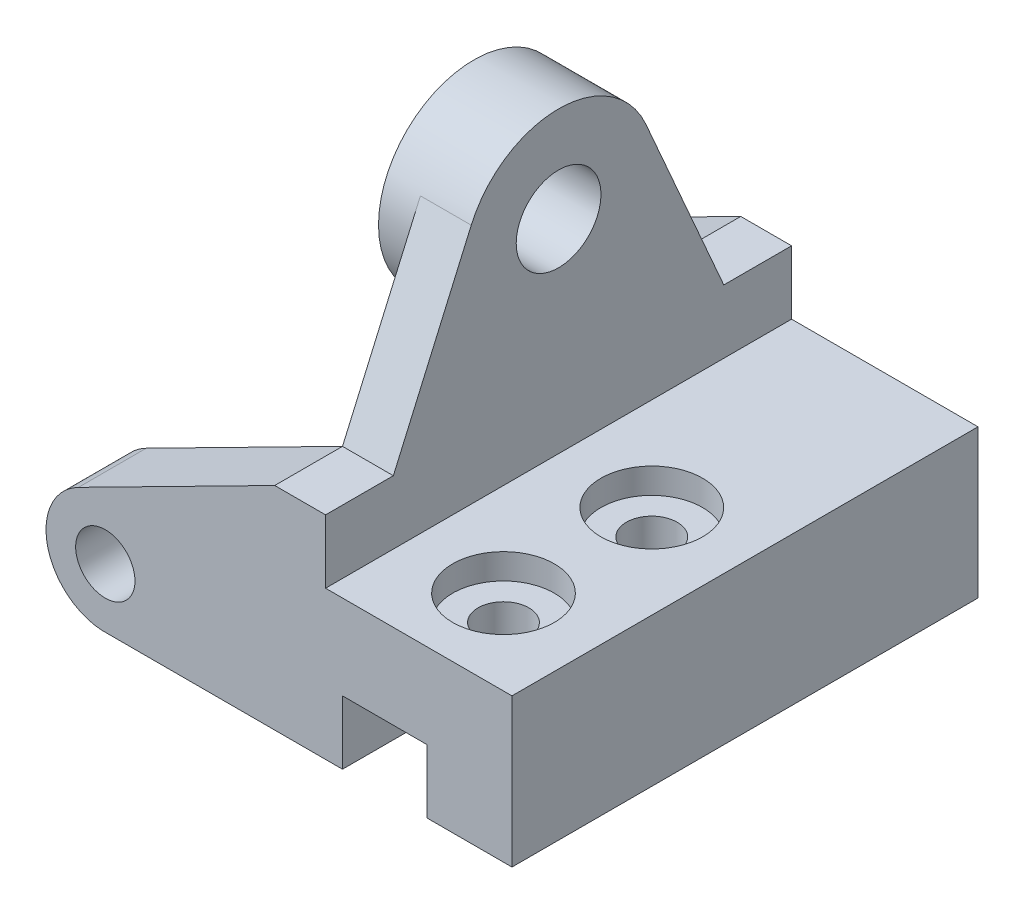
ISO-10303-21;
HEADER;
FILE_DESCRIPTION(('STEP AP214'),'2;1');
FILE_NAME('part.step','',(''),(''),'','','');
FILE_SCHEMA(('AUTOMOTIVE_DESIGN { 1 0 10303 214 1 1 1 1 }'));
ENDSEC;
DATA;
#1=APPLICATION_CONTEXT('core data for automotive mechanical design processes');
#2=APPLICATION_PROTOCOL_DEFINITION('international standard','automotive_design',2000,#1);
#3=PRODUCT_CONTEXT('',#1,'mechanical');
#4=PRODUCT('Part','Part','',(#3));
#5=PRODUCT_RELATED_PRODUCT_CATEGORY('part','',(#4));
#6=PRODUCT_DEFINITION_FORMATION('','',#4);
#7=PRODUCT_DEFINITION_CONTEXT('part definition',#1,'design');
#8=PRODUCT_DEFINITION('design','',#6,#7);
#9=PRODUCT_DEFINITION_SHAPE('','',#8);
#10=(LENGTH_UNIT() NAMED_UNIT(*) SI_UNIT(.MILLI.,.METRE.));
#11=(NAMED_UNIT(*) PLANE_ANGLE_UNIT() SI_UNIT($,.RADIAN.));
#12=(NAMED_UNIT(*) SI_UNIT($,.STERADIAN.) SOLID_ANGLE_UNIT());
#13=UNCERTAINTY_MEASURE_WITH_UNIT(LENGTH_MEASURE(1.E-05),#10,'distance_accuracy_value','');
#14=(GEOMETRIC_REPRESENTATION_CONTEXT(3) GLOBAL_UNCERTAINTY_ASSIGNED_CONTEXT((#13)) GLOBAL_UNIT_ASSIGNED_CONTEXT((#10,
#11,#12)) REPRESENTATION_CONTEXT('',''));
#15=CARTESIAN_POINT('',(0.,0.,0.));
#16=DIRECTION('',(0.,0.,1.));
#17=DIRECTION('',(1.,0.,0.));
#18=AXIS2_PLACEMENT_3D('',#15,#16,#17);
#19=CARTESIAN_POINT('',(6.,50.,0.));
#20=DIRECTION('',(0.,1.,0.));
#21=DIRECTION('',(0.,0.,1.));
#22=AXIS2_PLACEMENT_3D('',#19,#20,#21);
#23=PLANE('',#22);
#24=DIRECTION('',(0.,0.,1.));
#25=VECTOR('',#24,1.);
#26=CARTESIAN_POINT('',(6.,50.,0.));
#27=LINE('',#26,#25);
#28=CARTESIAN_POINT('',(6.,50.,94.));
#29=VERTEX_POINT('',#28);
#30=CARTESIAN_POINT('',(6.,50.,110.));
#31=VERTEX_POINT('',#30);
#32=EDGE_CURVE('E347',#29,#31,#27,.T.);
#33=ORIENTED_EDGE('',*,*,#32,.F.);
#34=DIRECTION('',(-1.,0.,0.));
#35=VECTOR('',#34,1.);
#36=CARTESIAN_POINT('',(6.,50.,94.));
#37=LINE('',#36,#35);
#38=CARTESIAN_POINT('',(-6.,50.,94.));
#39=VERTEX_POINT('',#38);
#40=EDGE_CURVE('E262',#29,#39,#37,.T.);
#41=ORIENTED_EDGE('',*,*,#40,.T.);
#42=DIRECTION('',(0.,0.,1.));
#43=VECTOR('',#42,1.);
#44=CARTESIAN_POINT('',(-6.,50.,94.));
#45=LINE('',#44,#43);
#46=CARTESIAN_POINT('',(-6.,50.,110.));
#47=VERTEX_POINT('',#46);
#48=EDGE_CURVE('E325',#39,#47,#45,.T.);
#49=ORIENTED_EDGE('',*,*,#48,.T.);
#50=DIRECTION('',(-1.,0.,0.));
#51=VECTOR('',#50,1.);
#52=CARTESIAN_POINT('',(6.,50.,110.));
#53=LINE('',#52,#51);
#54=EDGE_CURVE('E332',#31,#47,#53,.T.);
#55=ORIENTED_EDGE('',*,*,#54,.F.);
#56=EDGE_LOOP('',(#33,#41,#49,#55));
#57=FACE_BOUND('',#56,.T.);
#58=ADVANCED_FACE('F50',(#57),#23,.T.);
#59=CARTESIAN_POINT('',(-6.,35.,110.));
#60=DIRECTION('',(1.,0.,0.));
#61=DIRECTION('',(0.,0.,-1.));
#62=AXIS2_PLACEMENT_3D('',#59,#60,#61);
#63=PLANE('',#62);
#64=CARTESIAN_POINT('',(-6.,83.,55.));
#65=DIRECTION('',(-1.,0.,0.));
#66=DIRECTION('',(0.,0.,1.));
#67=AXIS2_PLACEMENT_3D('',#64,#65,#66);
#68=CIRCLE('',#67,22.5);
#69=CARTESIAN_POINT('',(-6.,92.0198235139329,34.3870724112875));
#70=VERTEX_POINT('',#69);
#71=CARTESIAN_POINT('',(-6.,92.0198235139329,75.6129275887125));
#72=VERTEX_POINT('',#71);
#73=EDGE_CURVE('E240',#70,#72,#68,.T.);
#74=ORIENTED_EDGE('',*,*,#73,.F.);
#75=DIRECTION('',(0.,-0.916130115053887,-0.400881045063684));
#76=VECTOR('',#75,1.);
#77=CARTESIAN_POINT('',(-6.,92.0198235139329,34.3870724112875));
#78=LINE('',#77,#76);
#79=CARTESIAN_POINT('',(-6.,50.,16.));
#80=VERTEX_POINT('',#79);
#81=EDGE_CURVE('E243',#70,#80,#78,.T.);
#82=ORIENTED_EDGE('',*,*,#81,.T.);
#83=DIRECTION('',(0.,-1.,0.));
#84=VECTOR('',#83,1.);
#85=CARTESIAN_POINT('',(-6.,50.,16.));
#86=LINE('',#85,#84);
#87=CARTESIAN_POINT('',(-6.,0.,16.));
#88=VERTEX_POINT('',#87);
#89=EDGE_CURVE('E278',#80,#88,#86,.T.);
#90=ORIENTED_EDGE('',*,*,#89,.T.);
#91=DIRECTION('',(0.,0.,-1.));
#92=VECTOR('',#91,1.);
#93=CARTESIAN_POINT('',(-6.,0.,110.));
#94=LINE('',#93,#92);
#95=CARTESIAN_POINT('',(-6.,0.,94.));
#96=VERTEX_POINT('',#95);
#97=EDGE_CURVE('E390',#96,#88,#94,.T.);
#98=ORIENTED_EDGE('',*,*,#97,.F.);
#99=DIRECTION('',(0.,-1.,0.));
#100=VECTOR('',#99,1.);
#101=CARTESIAN_POINT('',(-6.,0.,94.));
#102=LINE('',#101,#100);
#103=EDGE_CURVE('E313',#39,#96,#102,.T.);
#104=ORIENTED_EDGE('',*,*,#103,.F.);
#105=DIRECTION('',(0.,0.916130115053887,-0.400881045063683));
#106=VECTOR('',#105,1.);
#107=CARTESIAN_POINT('',(-6.,50.,94.));
#108=LINE('',#107,#106);
#109=EDGE_CURVE('E249',#39,#72,#108,.T.);
#110=ORIENTED_EDGE('',*,*,#109,.T.);
#111=EDGE_LOOP('',(#74,#82,#90,#98,#104,#110));
#112=FACE_BOUND('',#111,.T.);
#113=ADVANCED_FACE('F475',(#112),#63,.F.);
#114=CARTESIAN_POINT('',(-6.,0.,110.));
#115=DIRECTION('',(0.,1.,0.));
#116=DIRECTION('',(0.,0.,1.));
#117=AXIS2_PLACEMENT_3D('',#114,#115,#116);
#118=PLANE('',#117);
#119=DIRECTION('',(0.,0.,1.));
#120=VECTOR('',#119,1.);
#121=CARTESIAN_POINT('',(30.,0.,0.));
#122=LINE('',#121,#120);
#123=CARTESIAN_POINT('',(30.,0.,0.));
#124=VERTEX_POINT('',#123);
#125=CARTESIAN_POINT('',(30.,0.,110.));
#126=VERTEX_POINT('',#125);
#127=EDGE_CURVE('E366',#124,#126,#122,.T.);
#128=ORIENTED_EDGE('',*,*,#127,.F.);
#129=DIRECTION('',(1.,0.,0.));
#130=VECTOR('',#129,1.);
#131=CARTESIAN_POINT('',(-6.,0.,0.));
#132=LINE('',#131,#130);
#133=CARTESIAN_POINT('',(50.,0.,0.));
#134=VERTEX_POINT('',#133);
#135=EDGE_CURVE('E368',#124,#134,#132,.T.);
#136=ORIENTED_EDGE('',*,*,#135,.T.);
#137=DIRECTION('',(0.,0.,-1.));
#138=VECTOR('',#137,1.);
#139=CARTESIAN_POINT('',(50.,0.,110.));
#140=LINE('',#139,#138);
#141=CARTESIAN_POINT('',(50.,0.,110.));
#142=VERTEX_POINT('',#141);
#143=EDGE_CURVE('E402',#142,#134,#140,.T.);
#144=ORIENTED_EDGE('',*,*,#143,.F.);
#145=DIRECTION('',(1.,0.,0.));
#146=VECTOR('',#145,1.);
#147=CARTESIAN_POINT('',(-6.,0.,110.));
#148=LINE('',#147,#146);
#149=EDGE_CURVE('E385',#126,#142,#148,.T.);
#150=ORIENTED_EDGE('',*,*,#149,.F.);
#151=EDGE_LOOP('',(#128,#136,#144,#150));
#152=FACE_BOUND('',#151,.T.);
#153=ADVANCED_FACE('F47',(#152),#118,.F.);
#154=DIRECTION('',(0.,0.,1.));
#155=VECTOR('',#154,1.);
#156=CARTESIAN_POINT('',(10.,0.,0.));
#157=LINE('',#156,#155);
#158=CARTESIAN_POINT('',(10.,0.,0.));
#159=VERTEX_POINT('',#158);
#160=CARTESIAN_POINT('',(10.,0.,110.));
#161=VERTEX_POINT('',#160);
#162=EDGE_CURVE('E367',#159,#161,#157,.T.);
#163=ORIENTED_EDGE('',*,*,#162,.T.);
#164=CARTESIAN_POINT('',(-45.1510571856392,0.,110.));
#165=VERTEX_POINT('',#164);
#166=EDGE_CURVE('E377',#165,#161,#148,.T.);
#167=ORIENTED_EDGE('',*,*,#166,.F.);
#168=DIRECTION('',(0.,0.,1.));
#169=VECTOR('',#168,1.);
#170=CARTESIAN_POINT('',(-45.1510571856392,0.,94.));
#171=LINE('',#170,#169);
#172=CARTESIAN_POINT('',(-45.1510571856392,0.,94.));
#173=VERTEX_POINT('',#172);
#174=EDGE_CURVE('E324',#173,#165,#171,.T.);
#175=ORIENTED_EDGE('',*,*,#174,.F.);
#176=DIRECTION('',(-1.,0.,0.));
#177=VECTOR('',#176,1.);
#178=CARTESIAN_POINT('',(0.,0.,94.));
#179=LINE('',#178,#177);
#180=EDGE_CURVE('E315',#96,#173,#179,.T.);
#181=ORIENTED_EDGE('',*,*,#180,.F.);
#182=ORIENTED_EDGE('',*,*,#97,.T.);
#183=DIRECTION('',(-1.,0.,0.));
#184=VECTOR('',#183,1.);
#185=CARTESIAN_POINT('',(-6.,0.,16.));
#186=LINE('',#185,#184);
#187=CARTESIAN_POINT('',(-45.1510571856392,0.,16.));
#188=VERTEX_POINT('',#187);
#189=EDGE_CURVE('E282',#88,#188,#186,.T.);
#190=ORIENTED_EDGE('',*,*,#189,.T.);
#191=DIRECTION('',(0.,0.,-1.));
#192=VECTOR('',#191,1.);
#193=CARTESIAN_POINT('',(-45.1510571856392,0.,16.));
#194=LINE('',#193,#192);
#195=CARTESIAN_POINT('',(-45.1510571856392,0.,0.));
#196=VERTEX_POINT('',#195);
#197=EDGE_CURVE('E290',#188,#196,#194,.T.);
#198=ORIENTED_EDGE('',*,*,#197,.T.);
#199=EDGE_CURVE('E387',#196,#159,#132,.T.);
#200=ORIENTED_EDGE('',*,*,#199,.T.);
#201=EDGE_LOOP('',(#163,#167,#175,#181,#182,#190,#198,#200));
#202=FACE_BOUND('',#201,.T.);
#203=ADVANCED_FACE('F456',(#202),#118,.F.);
#204=CARTESIAN_POINT('',(0.,0.,110.));
#205=DIRECTION('',(0.,0.,1.));
#206=DIRECTION('',(1.,0.,0.));
#207=AXIS2_PLACEMENT_3D('',#204,#205,#206);
#208=PLANE('',#207);
#209=CARTESIAN_POINT('',(-45.9872968007716,13.9750028016485,110.));
#210=DIRECTION('',(0.,0.,1.));
#211=DIRECTION('',(1.,0.,0.));
#212=AXIS2_PLACEMENT_3D('',#209,#210,#211);
#213=CIRCLE('',#212,7.);
#214=CARTESIAN_POINT('',(-38.9872968007716,13.9750028016485,110.));
#215=VERTEX_POINT('',#214);
#216=EDGE_CURVE('E298',#215,#215,#213,.T.);
#217=ORIENTED_EDGE('',*,*,#216,.F.);
#218=EDGE_LOOP('',(#217));
#219=FACE_BOUND('',#218,.T.);
#220=DIRECTION('',(1.,0.,0.));
#221=VECTOR('',#220,1.);
#222=CARTESIAN_POINT('',(0.,15.,110.));
#223=LINE('',#222,#221);
#224=CARTESIAN_POINT('',(10.,15.,110.));
#225=VERTEX_POINT('',#224);
#226=CARTESIAN_POINT('',(30.,15.,110.));
#227=VERTEX_POINT('',#226);
#228=EDGE_CURVE('E363',#225,#227,#223,.T.);
#229=ORIENTED_EDGE('',*,*,#228,.T.);
#230=DIRECTION('',(0.,-1.,0.));
#231=VECTOR('',#230,1.);
#232=CARTESIAN_POINT('',(30.,0.,110.));
#233=LINE('',#232,#231);
#234=EDGE_CURVE('E343',#227,#126,#233,.T.);
#235=ORIENTED_EDGE('',*,*,#234,.T.);
#236=ORIENTED_EDGE('',*,*,#149,.T.);
#237=DIRECTION('',(0.,1.,0.));
#238=VECTOR('',#237,1.);
#239=CARTESIAN_POINT('',(50.,0.,110.));
#240=LINE('',#239,#238);
#241=CARTESIAN_POINT('',(50.,35.,110.));
#242=VERTEX_POINT('',#241);
#243=EDGE_CURVE('E382',#142,#242,#240,.T.);
#244=ORIENTED_EDGE('',*,*,#243,.T.);
#245=DIRECTION('',(-1.,0.,0.));
#246=VECTOR('',#245,1.);
#247=CARTESIAN_POINT('',(-6.,35.,110.));
#248=LINE('',#247,#246);
#249=CARTESIAN_POINT('',(6.,35.,110.));
#250=VERTEX_POINT('',#249);
#251=EDGE_CURVE('E381',#242,#250,#248,.T.);
#252=ORIENTED_EDGE('',*,*,#251,.T.);
#253=DIRECTION('',(0.,1.,0.));
#254=VECTOR('',#253,1.);
#255=CARTESIAN_POINT('',(6.,35.,110.));
#256=LINE('',#255,#254);
#257=EDGE_CURVE('E323',#250,#31,#256,.T.);
#258=ORIENTED_EDGE('',*,*,#257,.T.);
#259=ORIENTED_EDGE('',*,*,#54,.T.);
#260=DIRECTION('',(-0.891489434409362,-0.45304148633042,0.));
#261=VECTOR('',#260,1.);
#262=CARTESIAN_POINT('',(-21.425564450653,42.1609607736523,110.));
#263=LINE('',#262,#261);
#264=CARTESIAN_POINT('',(-52.3298776093975,26.4558548833796,110.));
#265=VERTEX_POINT('',#264);
#266=EDGE_CURVE('E305',#47,#265,#263,.T.);
#267=ORIENTED_EDGE('',*,*,#266,.T.);
#268=CARTESIAN_POINT('',(-45.9872968007716,13.9750028016485,110.));
#269=DIRECTION('',(0.,0.,1.));
#270=DIRECTION('',(1.,0.,0.));
#271=AXIS2_PLACEMENT_3D('',#268,#269,#270);
#272=CIRCLE('',#271,14.);
#273=EDGE_CURVE('E307',#265,#165,#272,.T.);
#274=ORIENTED_EDGE('',*,*,#273,.T.);
#275=ORIENTED_EDGE('',*,*,#166,.T.);
#276=DIRECTION('',(0.,1.,0.));
#277=VECTOR('',#276,1.);
#278=CARTESIAN_POINT('',(10.,0.,110.));
#279=LINE('',#278,#277);
#280=EDGE_CURVE('E355',#161,#225,#279,.T.);
#281=ORIENTED_EDGE('',*,*,#280,.T.);
#282=EDGE_LOOP('',(#229,#235,#236,#244,#252,#258,#259,#267,#274,#275,#281));
#283=FACE_BOUND('',#282,.T.);
#284=ADVANCED_FACE('F429',(#219,#283),#208,.T.);
#285=CARTESIAN_POINT('',(0.,0.,0.));
#286=DIRECTION('',(0.,0.,1.));
#287=DIRECTION('',(1.,0.,0.));
#288=AXIS2_PLACEMENT_3D('',#285,#286,#287);
#289=PLANE('',#288);
#290=CARTESIAN_POINT('',(-45.9872968007716,13.9750028016485,0.));
#291=DIRECTION('',(0.,0.,-1.));
#292=DIRECTION('',(-1.,0.,0.));
#293=AXIS2_PLACEMENT_3D('',#290,#291,#292);
#294=CIRCLE('',#293,7.);
#295=CARTESIAN_POINT('',(-52.9872968007716,13.9750028016485,0.));
#296=VERTEX_POINT('',#295);
#297=EDGE_CURVE('E265',#296,#296,#294,.T.);
#298=ORIENTED_EDGE('',*,*,#297,.F.);
#299=EDGE_LOOP('',(#298));
#300=FACE_BOUND('',#299,.T.);
#301=DIRECTION('',(0.,-1.,0.));
#302=VECTOR('',#301,1.);
#303=CARTESIAN_POINT('',(30.,0.,0.));
#304=LINE('',#303,#302);
#305=CARTESIAN_POINT('',(30.,15.,0.));
#306=VERTEX_POINT('',#305);
#307=EDGE_CURVE('E353',#306,#124,#304,.T.);
#308=ORIENTED_EDGE('',*,*,#307,.F.);
#309=DIRECTION('',(1.,0.,0.));
#310=VECTOR('',#309,1.);
#311=CARTESIAN_POINT('',(0.,15.,0.));
#312=LINE('',#311,#310);
#313=CARTESIAN_POINT('',(10.,15.,0.));
#314=VERTEX_POINT('',#313);
#315=EDGE_CURVE('E352',#314,#306,#312,.T.);
#316=ORIENTED_EDGE('',*,*,#315,.F.);
#317=DIRECTION('',(0.,1.,0.));
#318=VECTOR('',#317,1.);
#319=CARTESIAN_POINT('',(10.,0.,0.));
#320=LINE('',#319,#318);
#321=EDGE_CURVE('E358',#159,#314,#320,.T.);
#322=ORIENTED_EDGE('',*,*,#321,.F.);
#323=ORIENTED_EDGE('',*,*,#199,.F.);
#324=CARTESIAN_POINT('',(-45.9872968007716,13.9750028016485,0.));
#325=DIRECTION('',(0.,0.,-1.));
#326=DIRECTION('',(-1.,0.,0.));
#327=AXIS2_PLACEMENT_3D('',#324,#325,#326);
#328=CIRCLE('',#327,14.);
#329=CARTESIAN_POINT('',(-52.3298776093975,26.4558548833796,0.));
#330=VERTEX_POINT('',#329);
#331=EDGE_CURVE('E279',#196,#330,#328,.T.);
#332=ORIENTED_EDGE('',*,*,#331,.T.);
#333=DIRECTION('',(0.891489434409362,0.45304148633042,0.));
#334=VECTOR('',#333,1.);
#335=CARTESIAN_POINT('',(-6.,50.,0.));
#336=LINE('',#335,#334);
#337=CARTESIAN_POINT('',(-6.,50.,0.));
#338=VERTEX_POINT('',#337);
#339=EDGE_CURVE('E271',#330,#338,#336,.T.);
#340=ORIENTED_EDGE('',*,*,#339,.T.);
#341=DIRECTION('',(-1.,0.,0.));
#342=VECTOR('',#341,1.);
#343=CARTESIAN_POINT('',(6.,50.,0.));
#344=LINE('',#343,#342);
#345=CARTESIAN_POINT('',(6.,50.,0.));
#346=VERTEX_POINT('',#345);
#347=EDGE_CURVE('E334',#346,#338,#344,.T.);
#348=ORIENTED_EDGE('',*,*,#347,.F.);
#349=DIRECTION('',(0.,1.,0.));
#350=VECTOR('',#349,1.);
#351=CARTESIAN_POINT('',(6.,35.,0.));
#352=LINE('',#351,#350);
#353=CARTESIAN_POINT('',(6.,35.,0.));
#354=VERTEX_POINT('',#353);
#355=EDGE_CURVE('E328',#354,#346,#352,.T.);
#356=ORIENTED_EDGE('',*,*,#355,.F.);
#357=DIRECTION('',(-1.,0.,0.));
#358=VECTOR('',#357,1.);
#359=CARTESIAN_POINT('',(-6.,35.,0.));
#360=LINE('',#359,#358);
#361=CARTESIAN_POINT('',(50.,35.,0.));
#362=VERTEX_POINT('',#361);
#363=EDGE_CURVE('E392',#362,#354,#360,.T.);
#364=ORIENTED_EDGE('',*,*,#363,.F.);
#365=DIRECTION('',(0.,1.,0.));
#366=VECTOR('',#365,1.);
#367=CARTESIAN_POINT('',(50.,0.,0.));
#368=LINE('',#367,#366);
#369=EDGE_CURVE('E391',#134,#362,#368,.T.);
#370=ORIENTED_EDGE('',*,*,#369,.F.);
#371=ORIENTED_EDGE('',*,*,#135,.F.);
#372=EDGE_LOOP('',(#308,#316,#322,#323,#332,#340,#348,#356,#364,#370,#371));
#373=FACE_BOUND('',#372,.T.);
#374=ADVANCED_FACE('F416',(#300,#373),#289,.F.);
#375=CARTESIAN_POINT('',(50.,0.,110.));
#376=DIRECTION('',(-1.,0.,0.));
#377=DIRECTION('',(0.,0.,1.));
#378=AXIS2_PLACEMENT_3D('',#375,#376,#377);
#379=PLANE('',#378);
#380=ORIENTED_EDGE('',*,*,#369,.T.);
#381=DIRECTION('',(0.,0.,-1.));
#382=VECTOR('',#381,1.);
#383=CARTESIAN_POINT('',(50.,35.,110.));
#384=LINE('',#383,#382);
#385=EDGE_CURVE('E397',#242,#362,#384,.T.);
#386=ORIENTED_EDGE('',*,*,#385,.F.);
#387=ORIENTED_EDGE('',*,*,#243,.F.);
#388=ORIENTED_EDGE('',*,*,#143,.T.);
#389=EDGE_LOOP('',(#380,#386,#387,#388));
#390=FACE_BOUND('',#389,.T.);
#391=ADVANCED_FACE('F435',(#390),#379,.F.);
#392=CARTESIAN_POINT('',(-6.,35.,110.));
#393=DIRECTION('',(0.,-1.,0.));
#394=DIRECTION('',(0.,0.,-1.));
#395=AXIS2_PLACEMENT_3D('',#392,#393,#394);
#396=PLANE('',#395);
#397=CARTESIAN_POINT('',(28.,35.,55.));
#398=DIRECTION('',(0.,1.,0.));
#399=DIRECTION('',(0.,0.,1.));
#400=AXIS2_PLACEMENT_3D('',#397,#398,#399);
#401=CIRCLE('',#400,12.);
#402=CARTESIAN_POINT('',(28.,35.,67.));
#403=VERTEX_POINT('',#402);
#404=EDGE_CURVE('E228',#403,#403,#401,.T.);
#405=ORIENTED_EDGE('',*,*,#404,.F.);
#406=EDGE_LOOP('',(#405));
#407=FACE_BOUND('',#406,.T.);
#408=CARTESIAN_POINT('',(28.,35.,90.));
#409=DIRECTION('',(0.,1.,0.));
#410=DIRECTION('',(0.,0.,1.));
#411=AXIS2_PLACEMENT_3D('',#408,#409,#410);
#412=CIRCLE('',#411,12.);
#413=CARTESIAN_POINT('',(28.,35.,102.));
#414=VERTEX_POINT('',#413);
#415=EDGE_CURVE('E223',#414,#414,#412,.T.);
#416=ORIENTED_EDGE('',*,*,#415,.F.);
#417=EDGE_LOOP('',(#416));
#418=FACE_BOUND('',#417,.T.);
#419=ORIENTED_EDGE('',*,*,#363,.T.);
#420=DIRECTION('',(0.,0.,1.));
#421=VECTOR('',#420,1.);
#422=CARTESIAN_POINT('',(6.,35.,0.));
#423=LINE('',#422,#421);
#424=EDGE_CURVE('E337',#354,#250,#423,.T.);
#425=ORIENTED_EDGE('',*,*,#424,.T.);
#426=ORIENTED_EDGE('',*,*,#251,.F.);
#427=ORIENTED_EDGE('',*,*,#385,.T.);
#428=EDGE_LOOP('',(#419,#425,#426,#427));
#429=FACE_BOUND('',#428,.T.);
#430=ADVANCED_FACE('F436',(#407,#418,#429),#396,.F.);
#431=CARTESIAN_POINT('',(30.,0.,0.));
#432=DIRECTION('',(-1.,0.,0.));
#433=DIRECTION('',(0.,0.,1.));
#434=AXIS2_PLACEMENT_3D('',#431,#432,#433);
#435=PLANE('',#434);
#436=DIRECTION('',(0.,1.,0.));
#437=VECTOR('',#436,1.);
#438=CARTESIAN_POINT('',(30.,9.,60.6568542494924));
#439=LINE('',#438,#437);
#440=CARTESIAN_POINT('',(30.,9.,60.6568542494924));
#441=VERTEX_POINT('',#440);
#442=CARTESIAN_POINT('',(30.,15.,60.6568542494924));
#443=VERTEX_POINT('',#442);
#444=EDGE_CURVE('E69',#441,#443,#439,.T.);
#445=ORIENTED_EDGE('',*,*,#444,.F.);
#446=DIRECTION('',(0.,0.,-1.));
#447=VECTOR('',#446,1.);
#448=CARTESIAN_POINT('',(30.,9.,0.));
#449=LINE('',#448,#447);
#450=CARTESIAN_POINT('',(30.,9.,49.3431457505076));
#451=VERTEX_POINT('',#450);
#452=EDGE_CURVE('E11',#441,#451,#449,.T.);
#453=ORIENTED_EDGE('',*,*,#452,.T.);
#454=DIRECTION('',(0.,1.,0.));
#455=VECTOR('',#454,1.);
#456=CARTESIAN_POINT('',(30.,9.,49.3431457505076));
#457=LINE('',#456,#455);
#458=CARTESIAN_POINT('',(30.,15.,49.3431457505076));
#459=VERTEX_POINT('',#458);
#460=EDGE_CURVE('E212',#459,#451,#457,.F.);
#461=ORIENTED_EDGE('',*,*,#460,.F.);
#462=DIRECTION('',(0.,0.,1.));
#463=VECTOR('',#462,1.);
#464=CARTESIAN_POINT('',(30.,15.,0.));
#465=LINE('',#464,#463);
#466=EDGE_CURVE('E372',#306,#459,#465,.T.);
#467=ORIENTED_EDGE('',*,*,#466,.F.);
#468=ORIENTED_EDGE('',*,*,#307,.T.);
#469=ORIENTED_EDGE('',*,*,#127,.T.);
#470=ORIENTED_EDGE('',*,*,#234,.F.);
#471=CARTESIAN_POINT('',(30.,15.,95.6568542494924));
#472=VERTEX_POINT('',#471);
#473=EDGE_CURVE('E215',#472,#227,#465,.T.);
#474=ORIENTED_EDGE('',*,*,#473,.F.);
#475=DIRECTION('',(0.,1.,0.));
#476=VECTOR('',#475,1.);
#477=CARTESIAN_POINT('',(30.,9.,95.6568542494924));
#478=LINE('',#477,#476);
#479=CARTESIAN_POINT('',(30.,9.,95.6568542494924));
#480=VERTEX_POINT('',#479);
#481=EDGE_CURVE('E65',#480,#472,#478,.T.);
#482=ORIENTED_EDGE('',*,*,#481,.F.);
#483=DIRECTION('',(0.,0.,-1.));
#484=VECTOR('',#483,1.);
#485=CARTESIAN_POINT('',(30.,9.,0.));
#486=LINE('',#485,#484);
#487=CARTESIAN_POINT('',(30.,9.,84.3431457505076));
#488=VERTEX_POINT('',#487);
#489=EDGE_CURVE('E54',#480,#488,#486,.T.);
#490=ORIENTED_EDGE('',*,*,#489,.T.);
#491=DIRECTION('',(0.,1.,0.));
#492=VECTOR('',#491,1.);
#493=CARTESIAN_POINT('',(30.,9.,84.3431457505076));
#494=LINE('',#493,#492);
#495=CARTESIAN_POINT('',(30.,15.,84.3431457505076));
#496=VERTEX_POINT('',#495);
#497=EDGE_CURVE('E201',#496,#488,#494,.F.);
#498=ORIENTED_EDGE('',*,*,#497,.F.);
#499=EDGE_CURVE('E380',#443,#496,#465,.T.);
#500=ORIENTED_EDGE('',*,*,#499,.F.);
#501=EDGE_LOOP('',(#445,#453,#461,#467,#468,#469,#470,#474,#482,#490,#498,#500));
#502=FACE_BOUND('',#501,.T.);
#503=ADVANCED_FACE('F208',(#502),#435,.T.);
#504=CARTESIAN_POINT('',(10.,0.,0.));
#505=DIRECTION('',(1.,0.,0.));
#506=DIRECTION('',(0.,0.,-1.));
#507=AXIS2_PLACEMENT_3D('',#504,#505,#506);
#508=PLANE('',#507);
#509=ORIENTED_EDGE('',*,*,#280,.F.);
#510=ORIENTED_EDGE('',*,*,#162,.F.);
#511=ORIENTED_EDGE('',*,*,#321,.T.);
#512=DIRECTION('',(0.,0.,1.));
#513=VECTOR('',#512,1.);
#514=CARTESIAN_POINT('',(10.,15.,0.));
#515=LINE('',#514,#513);
#516=EDGE_CURVE('E375',#314,#225,#515,.T.);
#517=ORIENTED_EDGE('',*,*,#516,.T.);
#518=EDGE_LOOP('',(#509,#510,#511,#517));
#519=FACE_BOUND('',#518,.T.);
#520=ADVANCED_FACE('F457',(#519),#508,.T.);
#521=CARTESIAN_POINT('',(0.,15.,0.));
#522=DIRECTION('',(0.,-1.,0.));
#523=DIRECTION('',(0.,0.,-1.));
#524=AXIS2_PLACEMENT_3D('',#521,#522,#523);
#525=PLANE('',#524);
#526=CARTESIAN_POINT('',(28.,15.,55.));
#527=DIRECTION('',(0.,-1.,0.));
#528=DIRECTION('',(0.,0.,-1.));
#529=AXIS2_PLACEMENT_3D('',#526,#527,#528);
#530=CIRCLE('',#529,6.);
#531=EDGE_CURVE('E204',#443,#459,#530,.T.);
#532=ORIENTED_EDGE('',*,*,#531,.F.);
#533=ORIENTED_EDGE('',*,*,#499,.T.);
#534=CARTESIAN_POINT('',(28.,15.,90.));
#535=DIRECTION('',(0.,-1.,0.));
#536=DIRECTION('',(0.,0.,-1.));
#537=AXIS2_PLACEMENT_3D('',#534,#535,#536);
#538=CIRCLE('',#537,6.00000000000001);
#539=EDGE_CURVE('E404',#472,#496,#538,.T.);
#540=ORIENTED_EDGE('',*,*,#539,.F.);
#541=ORIENTED_EDGE('',*,*,#473,.T.);
#542=ORIENTED_EDGE('',*,*,#228,.F.);
#543=ORIENTED_EDGE('',*,*,#516,.F.);
#544=ORIENTED_EDGE('',*,*,#315,.T.);
#545=ORIENTED_EDGE('',*,*,#466,.T.);
#546=EDGE_LOOP('',(#532,#533,#540,#541,#542,#543,#544,#545));
#547=FACE_BOUND('',#546,.T.);
#548=ADVANCED_FACE('F414',(#547),#525,.T.);
#549=DIRECTION('',(-1.,0.,0.));
#550=VECTOR('',#549,1.);
#551=CARTESIAN_POINT('',(6.,50.,16.));
#552=LINE('',#551,#550);
#553=CARTESIAN_POINT('',(6.,50.,16.));
#554=VERTEX_POINT('',#553);
#555=EDGE_CURVE('E268',#554,#80,#552,.T.);
#556=ORIENTED_EDGE('',*,*,#555,.F.);
#557=EDGE_CURVE('E344',#346,#554,#27,.T.);
#558=ORIENTED_EDGE('',*,*,#557,.F.);
#559=ORIENTED_EDGE('',*,*,#347,.T.);
#560=DIRECTION('',(0.,0.,1.));
#561=VECTOR('',#560,1.);
#562=CARTESIAN_POINT('',(-6.,50.,0.));
#563=LINE('',#562,#561);
#564=EDGE_CURVE('E341',#338,#80,#563,.T.);
#565=ORIENTED_EDGE('',*,*,#564,.T.);
#566=EDGE_LOOP('',(#556,#558,#559,#565));
#567=FACE_BOUND('',#566,.T.);
#568=ADVANCED_FACE('F467',(#567),#23,.T.);
#569=CARTESIAN_POINT('',(6.,35.,0.));
#570=DIRECTION('',(1.,0.,0.));
#571=DIRECTION('',(0.,0.,-1.));
#572=AXIS2_PLACEMENT_3D('',#569,#570,#571);
#573=PLANE('',#572);
#574=CARTESIAN_POINT('',(6.,83.,55.));
#575=DIRECTION('',(-1.,0.,0.));
#576=DIRECTION('',(0.,0.,1.));
#577=AXIS2_PLACEMENT_3D('',#574,#575,#576);
#578=CIRCLE('',#577,10.);
#579=CARTESIAN_POINT('',(6.,83.,65.));
#580=VERTEX_POINT('',#579);
#581=EDGE_CURVE('E234',#580,#580,#578,.T.);
#582=ORIENTED_EDGE('',*,*,#581,.T.);
#583=EDGE_LOOP('',(#582));
#584=FACE_BOUND('',#583,.T.);
#585=ORIENTED_EDGE('',*,*,#257,.F.);
#586=ORIENTED_EDGE('',*,*,#424,.F.);
#587=ORIENTED_EDGE('',*,*,#355,.T.);
#588=ORIENTED_EDGE('',*,*,#557,.T.);
#589=DIRECTION('',(0.,-0.916130115053887,-0.400881045063684));
#590=VECTOR('',#589,1.);
#591=CARTESIAN_POINT('',(6.,92.0198235139329,34.3870724112875));
#592=LINE('',#591,#590);
#593=CARTESIAN_POINT('',(6.,92.0198235139329,34.3870724112875));
#594=VERTEX_POINT('',#593);
#595=EDGE_CURVE('E248',#594,#554,#592,.T.);
#596=ORIENTED_EDGE('',*,*,#595,.F.);
#597=CARTESIAN_POINT('',(6.,83.,55.));
#598=DIRECTION('',(-1.,0.,0.));
#599=DIRECTION('',(0.,0.,1.));
#600=AXIS2_PLACEMENT_3D('',#597,#598,#599);
#601=CIRCLE('',#600,22.5);
#602=CARTESIAN_POINT('',(6.,92.0198235139329,75.6129275887125));
#603=VERTEX_POINT('',#602);
#604=EDGE_CURVE('E246',#603,#594,#601,.T.);
#605=ORIENTED_EDGE('',*,*,#604,.F.);
#606=DIRECTION('',(0.,0.916130115053887,-0.400881045063683));
#607=VECTOR('',#606,1.);
#608=CARTESIAN_POINT('',(6.,50.,94.));
#609=LINE('',#608,#607);
#610=EDGE_CURVE('E255',#29,#603,#609,.T.);
#611=ORIENTED_EDGE('',*,*,#610,.F.);
#612=ORIENTED_EDGE('',*,*,#32,.T.);
#613=EDGE_LOOP('',(#585,#586,#587,#588,#596,#605,#611,#612));
#614=FACE_BOUND('',#613,.T.);
#615=ADVANCED_FACE('F484',(#584,#614),#573,.T.);
#616=CARTESIAN_POINT('',(-21.425564450653,42.1609607736523,94.));
#617=DIRECTION('',(-0.45304148633042,0.891489434409362,0.));
#618=DIRECTION('',(-0.891489434409362,-0.45304148633042,0.));
#619=AXIS2_PLACEMENT_3D('',#616,#617,#618);
#620=PLANE('',#619);
#621=ORIENTED_EDGE('',*,*,#266,.F.);
#622=ORIENTED_EDGE('',*,*,#48,.F.);
#623=DIRECTION('',(-0.891489434409362,-0.45304148633042,0.));
#624=VECTOR('',#623,1.);
#625=CARTESIAN_POINT('',(-21.425564450653,42.1609607736523,94.));
#626=LINE('',#625,#624);
#627=CARTESIAN_POINT('',(-52.3298776093975,26.4558548833796,94.));
#628=VERTEX_POINT('',#627);
#629=EDGE_CURVE('E304',#39,#628,#626,.T.);
#630=ORIENTED_EDGE('',*,*,#629,.T.);
#631=DIRECTION('',(0.,0.,1.));
#632=VECTOR('',#631,1.);
#633=CARTESIAN_POINT('',(-52.3298776093975,26.4558548833796,94.));
#634=LINE('',#633,#632);
#635=EDGE_CURVE('E320',#628,#265,#634,.T.);
#636=ORIENTED_EDGE('',*,*,#635,.T.);
#637=EDGE_LOOP('',(#621,#622,#630,#636));
#638=FACE_BOUND('',#637,.T.);
#639=ADVANCED_FACE('F447',(#638),#620,.T.);
#640=CARTESIAN_POINT('',(-45.9872968007716,13.9750028016485,94.));
#641=DIRECTION('',(0.,0.,1.));
#642=DIRECTION('',(1.,0.,0.));
#643=AXIS2_PLACEMENT_3D('',#640,#641,#642);
#644=CYLINDRICAL_SURFACE('',#643,14.);
#645=ORIENTED_EDGE('',*,*,#273,.F.);
#646=ORIENTED_EDGE('',*,*,#635,.F.);
#647=CARTESIAN_POINT('',(-45.9872968007716,13.9750028016485,94.));
#648=DIRECTION('',(0.,0.,1.));
#649=DIRECTION('',(1.,0.,0.));
#650=AXIS2_PLACEMENT_3D('',#647,#648,#649);
#651=CIRCLE('',#650,14.);
#652=EDGE_CURVE('E308',#628,#173,#651,.T.);
#653=ORIENTED_EDGE('',*,*,#652,.T.);
#654=ORIENTED_EDGE('',*,*,#174,.T.);
#655=EDGE_LOOP('',(#645,#646,#653,#654));
#656=FACE_BOUND('',#655,.T.);
#657=ADVANCED_FACE('F453',(#656),#644,.T.);
#658=CARTESIAN_POINT('',(0.,0.,94.));
#659=DIRECTION('',(0.,0.,1.));
#660=DIRECTION('',(1.,0.,0.));
#661=AXIS2_PLACEMENT_3D('',#658,#659,#660);
#662=PLANE('',#661);
#663=CARTESIAN_POINT('',(-45.9872968007716,13.9750028016485,94.));
#664=DIRECTION('',(0.,0.,1.));
#665=DIRECTION('',(1.,0.,0.));
#666=AXIS2_PLACEMENT_3D('',#663,#664,#665);
#667=CIRCLE('',#666,7.);
#668=CARTESIAN_POINT('',(-38.9872968007716,13.9750028016485,94.));
#669=VERTEX_POINT('',#668);
#670=EDGE_CURVE('E299',#669,#669,#667,.T.);
#671=ORIENTED_EDGE('',*,*,#670,.T.);
#672=EDGE_LOOP('',(#671));
#673=FACE_BOUND('',#672,.T.);
#674=ORIENTED_EDGE('',*,*,#629,.F.);
#675=ORIENTED_EDGE('',*,*,#103,.T.);
#676=ORIENTED_EDGE('',*,*,#180,.T.);
#677=ORIENTED_EDGE('',*,*,#652,.F.);
#678=EDGE_LOOP('',(#674,#675,#676,#677));
#679=FACE_BOUND('',#678,.T.);
#680=ADVANCED_FACE('F446',(#673,#679),#662,.F.);
#681=CARTESIAN_POINT('',(-45.9872968007716,13.9750028016485,94.));
#682=DIRECTION('',(0.,0.,1.));
#683=DIRECTION('',(1.,0.,0.));
#684=AXIS2_PLACEMENT_3D('',#681,#682,#683);
#685=CYLINDRICAL_SURFACE('',#684,7.);
#686=ORIENTED_EDGE('',*,*,#670,.F.);
#687=EDGE_LOOP('',(#686));
#688=FACE_BOUND('',#687,.T.);
#689=ORIENTED_EDGE('',*,*,#216,.T.);
#690=EDGE_LOOP('',(#689));
#691=FACE_BOUND('',#690,.T.);
#692=ADVANCED_FACE('F517',(#688,#691),#685,.F.);
#693=CARTESIAN_POINT('',(-6.,50.,16.));
#694=DIRECTION('',(-0.45304148633042,0.891489434409362,0.));
#695=DIRECTION('',(-0.891489434409362,-0.45304148633042,0.));
#696=AXIS2_PLACEMENT_3D('',#693,#694,#695);
#697=PLANE('',#696);
#698=ORIENTED_EDGE('',*,*,#339,.F.);
#699=DIRECTION('',(0.,0.,-1.));
#700=VECTOR('',#699,1.);
#701=CARTESIAN_POINT('',(-52.3298776093975,26.4558548833796,16.));
#702=LINE('',#701,#700);
#703=CARTESIAN_POINT('',(-52.3298776093975,26.4558548833796,16.));
#704=VERTEX_POINT('',#703);
#705=EDGE_CURVE('E295',#704,#330,#702,.T.);
#706=ORIENTED_EDGE('',*,*,#705,.F.);
#707=DIRECTION('',(0.891489434409362,0.45304148633042,0.));
#708=VECTOR('',#707,1.);
#709=CARTESIAN_POINT('',(-6.,50.,16.));
#710=LINE('',#709,#708);
#711=EDGE_CURVE('E276',#704,#80,#710,.T.);
#712=ORIENTED_EDGE('',*,*,#711,.T.);
#713=ORIENTED_EDGE('',*,*,#564,.F.);
#714=EDGE_LOOP('',(#698,#706,#712,#713));
#715=FACE_BOUND('',#714,.T.);
#716=ADVANCED_FACE('F498',(#715),#697,.T.);
#717=CARTESIAN_POINT('',(-45.9872968007716,13.9750028016485,16.));
#718=DIRECTION('',(0.,0.,-1.));
#719=DIRECTION('',(-1.,0.,0.));
#720=AXIS2_PLACEMENT_3D('',#717,#718,#719);
#721=CYLINDRICAL_SURFACE('',#720,14.);
#722=ORIENTED_EDGE('',*,*,#331,.F.);
#723=ORIENTED_EDGE('',*,*,#197,.F.);
#724=CARTESIAN_POINT('',(-45.9872968007716,13.9750028016485,16.));
#725=DIRECTION('',(0.,0.,-1.));
#726=DIRECTION('',(-1.,0.,0.));
#727=AXIS2_PLACEMENT_3D('',#724,#725,#726);
#728=CIRCLE('',#727,14.);
#729=EDGE_CURVE('E288',#188,#704,#728,.T.);
#730=ORIENTED_EDGE('',*,*,#729,.T.);
#731=ORIENTED_EDGE('',*,*,#705,.T.);
#732=EDGE_LOOP('',(#722,#723,#730,#731));
#733=FACE_BOUND('',#732,.T.);
#734=ADVANCED_FACE('F506',(#733),#721,.T.);
#735=CARTESIAN_POINT('',(-45.9872968007716,13.9750028016485,16.));
#736=DIRECTION('',(0.,0.,-1.));
#737=DIRECTION('',(-1.,0.,0.));
#738=AXIS2_PLACEMENT_3D('',#735,#736,#737);
#739=PLANE('',#738);
#740=CARTESIAN_POINT('',(-45.9872968007716,13.9750028016485,16.));
#741=DIRECTION('',(0.,0.,-1.));
#742=DIRECTION('',(-1.,0.,0.));
#743=AXIS2_PLACEMENT_3D('',#740,#741,#742);
#744=CIRCLE('',#743,7.);
#745=CARTESIAN_POINT('',(-52.9872968007716,13.9750028016485,16.));
#746=VERTEX_POINT('',#745);
#747=EDGE_CURVE('E266',#746,#746,#744,.T.);
#748=ORIENTED_EDGE('',*,*,#747,.T.);
#749=EDGE_LOOP('',(#748));
#750=FACE_BOUND('',#749,.T.);
#751=ORIENTED_EDGE('',*,*,#711,.F.);
#752=ORIENTED_EDGE('',*,*,#729,.F.);
#753=ORIENTED_EDGE('',*,*,#189,.F.);
#754=ORIENTED_EDGE('',*,*,#89,.F.);
#755=EDGE_LOOP('',(#751,#752,#753,#754));
#756=FACE_BOUND('',#755,.T.);
#757=ADVANCED_FACE('F503',(#750,#756),#739,.F.);
#758=CARTESIAN_POINT('',(-45.9872968007716,13.9750028016485,16.));
#759=DIRECTION('',(0.,0.,-1.));
#760=DIRECTION('',(-1.,0.,0.));
#761=AXIS2_PLACEMENT_3D('',#758,#759,#760);
#762=CYLINDRICAL_SURFACE('',#761,7.);
#763=ORIENTED_EDGE('',*,*,#747,.F.);
#764=EDGE_LOOP('',(#763));
#765=FACE_BOUND('',#764,.T.);
#766=ORIENTED_EDGE('',*,*,#297,.T.);
#767=EDGE_LOOP('',(#766));
#768=FACE_BOUND('',#767,.T.);
#769=ADVANCED_FACE('F511',(#765,#768),#762,.F.);
#770=CARTESIAN_POINT('',(6.,83.,55.));
#771=DIRECTION('',(-1.,0.,0.));
#772=DIRECTION('',(0.,0.,1.));
#773=AXIS2_PLACEMENT_3D('',#770,#771,#772);
#774=CYLINDRICAL_SURFACE('',#773,22.5);
#775=DIRECTION('',(-1.,0.,0.));
#776=VECTOR('',#775,1.);
#777=CARTESIAN_POINT('',(6.,92.0198235139329,34.3870724112875));
#778=LINE('',#777,#776);
#779=EDGE_CURVE('E253',#594,#70,#778,.T.);
#780=ORIENTED_EDGE('',*,*,#779,.T.);
#781=ORIENTED_EDGE('',*,*,#73,.T.);
#782=DIRECTION('',(-1.,0.,0.));
#783=VECTOR('',#782,1.);
#784=CARTESIAN_POINT('',(6.,92.0198235139329,75.6129275887125));
#785=LINE('',#784,#783);
#786=EDGE_CURVE('E259',#603,#72,#785,.T.);
#787=ORIENTED_EDGE('',*,*,#786,.F.);
#788=ORIENTED_EDGE('',*,*,#604,.T.);
#789=EDGE_LOOP('',(#780,#781,#787,#788));
#790=FACE_BOUND('',#789,.T.);
#791=CARTESIAN_POINT('',(-14.,83.,55.));
#792=DIRECTION('',(-1.,0.,0.));
#793=DIRECTION('',(0.,0.,1.));
#794=AXIS2_PLACEMENT_3D('',#791,#792,#793);
#795=CIRCLE('',#794,22.5);
#796=CARTESIAN_POINT('',(-14.,83.,77.5));
#797=VERTEX_POINT('',#796);
#798=EDGE_CURVE('E239',#797,#797,#795,.T.);
#799=ORIENTED_EDGE('',*,*,#798,.F.);
#800=EDGE_LOOP('',(#799));
#801=FACE_BOUND('',#800,.T.);
#802=ADVANCED_FACE('F572',(#790,#801),#774,.T.);
#803=CARTESIAN_POINT('',(6.,50.,94.));
#804=DIRECTION('',(0.,0.400881045063683,0.916130115053888));
#805=DIRECTION('',(0.,-0.916130115053888,0.400881045063683));
#806=AXIS2_PLACEMENT_3D('',#803,#804,#805);
#807=PLANE('',#806);
#808=ORIENTED_EDGE('',*,*,#109,.F.);
#809=ORIENTED_EDGE('',*,*,#40,.F.);
#810=ORIENTED_EDGE('',*,*,#610,.T.);
#811=ORIENTED_EDGE('',*,*,#786,.T.);
#812=EDGE_LOOP('',(#808,#809,#810,#811));
#813=FACE_BOUND('',#812,.T.);
#814=ADVANCED_FACE('F556',(#813),#807,.T.);
#815=CARTESIAN_POINT('',(6.,92.0198235139329,34.3870724112875));
#816=DIRECTION('',(0.,0.400881045063684,-0.916130115053887));
#817=DIRECTION('',(0.,0.916130115053887,0.400881045063684));
#818=AXIS2_PLACEMENT_3D('',#815,#816,#817);
#819=PLANE('',#818);
#820=ORIENTED_EDGE('',*,*,#81,.F.);
#821=ORIENTED_EDGE('',*,*,#779,.F.);
#822=ORIENTED_EDGE('',*,*,#595,.T.);
#823=ORIENTED_EDGE('',*,*,#555,.T.);
#824=EDGE_LOOP('',(#820,#821,#822,#823));
#825=FACE_BOUND('',#824,.T.);
#826=ADVANCED_FACE('F555',(#825),#819,.T.);
#827=CARTESIAN_POINT('',(-14.,83.,55.));
#828=DIRECTION('',(-1.,0.,0.));
#829=DIRECTION('',(0.,0.,1.));
#830=AXIS2_PLACEMENT_3D('',#827,#828,#829);
#831=PLANE('',#830);
#832=CARTESIAN_POINT('',(-14.,83.,55.));
#833=DIRECTION('',(-1.,0.,0.));
#834=DIRECTION('',(0.,0.,1.));
#835=AXIS2_PLACEMENT_3D('',#832,#833,#834);
#836=CIRCLE('',#835,10.);
#837=CARTESIAN_POINT('',(-14.,83.,65.));
#838=VERTEX_POINT('',#837);
#839=EDGE_CURVE('E221',#838,#838,#836,.T.);
#840=ORIENTED_EDGE('',*,*,#839,.F.);
#841=EDGE_LOOP('',(#840));
#842=FACE_BOUND('',#841,.T.);
#843=ORIENTED_EDGE('',*,*,#798,.T.);
#844=EDGE_LOOP('',(#843));
#845=FACE_BOUND('',#844,.T.);
#846=ADVANCED_FACE('F560',(#842,#845),#831,.T.);
#847=CARTESIAN_POINT('',(6.,83.,55.));
#848=DIRECTION('',(-1.,0.,0.));
#849=DIRECTION('',(0.,0.,1.));
#850=AXIS2_PLACEMENT_3D('',#847,#848,#849);
#851=CYLINDRICAL_SURFACE('',#850,10.);
#852=ORIENTED_EDGE('',*,*,#581,.F.);
#853=EDGE_LOOP('',(#852));
#854=FACE_BOUND('',#853,.T.);
#855=ORIENTED_EDGE('',*,*,#839,.T.);
#856=EDGE_LOOP('',(#855));
#857=FACE_BOUND('',#856,.T.);
#858=ADVANCED_FACE('F598',(#854,#857),#851,.F.);
#859=CARTESIAN_POINT('',(28.,29.,90.));
#860=DIRECTION('',(0.,1.,0.));
#861=DIRECTION('',(0.,0.,1.));
#862=AXIS2_PLACEMENT_3D('',#859,#860,#861);
#863=CYLINDRICAL_SURFACE('',#862,12.);
#864=CARTESIAN_POINT('',(28.,29.,90.));
#865=DIRECTION('',(0.,1.,0.));
#866=DIRECTION('',(0.,0.,1.));
#867=AXIS2_PLACEMENT_3D('',#864,#865,#866);
#868=CIRCLE('',#867,12.);
#869=CARTESIAN_POINT('',(28.,29.,102.));
#870=VERTEX_POINT('',#869);
#871=EDGE_CURVE('E230',#870,#870,#868,.T.);
#872=ORIENTED_EDGE('',*,*,#871,.F.);
#873=EDGE_LOOP('',(#872));
#874=FACE_BOUND('',#873,.T.);
#875=ORIENTED_EDGE('',*,*,#415,.T.);
#876=EDGE_LOOP('',(#875));
#877=FACE_BOUND('',#876,.T.);
#878=ADVANCED_FACE('F613',(#874,#877),#863,.F.);
#879=CARTESIAN_POINT('',(28.,29.,90.));
#880=DIRECTION('',(0.,1.,0.));
#881=DIRECTION('',(0.,0.,1.));
#882=AXIS2_PLACEMENT_3D('',#879,#880,#881);
#883=PLANE('',#882);
#884=CARTESIAN_POINT('',(28.,29.,90.));
#885=DIRECTION('',(0.,1.,0.));
#886=DIRECTION('',(0.,0.,1.));
#887=AXIS2_PLACEMENT_3D('',#884,#885,#886);
#888=CIRCLE('',#887,6.00000000000001);
#889=CARTESIAN_POINT('',(28.,29.,96.));
#890=VERTEX_POINT('',#889);
#891=EDGE_CURVE('E210',#890,#890,#888,.T.);
#892=ORIENTED_EDGE('',*,*,#891,.F.);
#893=EDGE_LOOP('',(#892));
#894=FACE_BOUND('',#893,.T.);
#895=ORIENTED_EDGE('',*,*,#871,.T.);
#896=EDGE_LOOP('',(#895));
#897=FACE_BOUND('',#896,.T.);
#898=ADVANCED_FACE('F631',(#894,#897),#883,.T.);
#899=CARTESIAN_POINT('',(28.,29.,55.));
#900=DIRECTION('',(0.,1.,0.));
#901=DIRECTION('',(0.,0.,1.));
#902=AXIS2_PLACEMENT_3D('',#899,#900,#901);
#903=CYLINDRICAL_SURFACE('',#902,12.);
#904=CARTESIAN_POINT('',(28.,29.,55.));
#905=DIRECTION('',(0.,1.,0.));
#906=DIRECTION('',(0.,0.,1.));
#907=AXIS2_PLACEMENT_3D('',#904,#905,#906);
#908=CIRCLE('',#907,12.);
#909=CARTESIAN_POINT('',(28.,29.,67.));
#910=VERTEX_POINT('',#909);
#911=EDGE_CURVE('E224',#910,#910,#908,.T.);
#912=ORIENTED_EDGE('',*,*,#911,.F.);
#913=EDGE_LOOP('',(#912));
#914=FACE_BOUND('',#913,.T.);
#915=ORIENTED_EDGE('',*,*,#404,.T.);
#916=EDGE_LOOP('',(#915));
#917=FACE_BOUND('',#916,.T.);
#918=ADVANCED_FACE('F637',(#914,#917),#903,.F.);
#919=CARTESIAN_POINT('',(28.,29.,55.));
#920=DIRECTION('',(0.,1.,0.));
#921=DIRECTION('',(0.,0.,1.));
#922=AXIS2_PLACEMENT_3D('',#919,#920,#921);
#923=PLANE('',#922);
#924=CARTESIAN_POINT('',(28.,29.,55.));
#925=DIRECTION('',(0.,1.,0.));
#926=DIRECTION('',(0.,0.,1.));
#927=AXIS2_PLACEMENT_3D('',#924,#925,#926);
#928=CIRCLE('',#927,6.);
#929=CARTESIAN_POINT('',(28.,29.,61.));
#930=VERTEX_POINT('',#929);
#931=EDGE_CURVE('E207',#930,#930,#928,.T.);
#932=ORIENTED_EDGE('',*,*,#931,.F.);
#933=EDGE_LOOP('',(#932));
#934=FACE_BOUND('',#933,.T.);
#935=ORIENTED_EDGE('',*,*,#911,.T.);
#936=EDGE_LOOP('',(#935));
#937=FACE_BOUND('',#936,.T.);
#938=ADVANCED_FACE('F642',(#934,#937),#923,.T.);
#939=CARTESIAN_POINT('',(28.,9.,90.));
#940=DIRECTION('',(0.,1.,0.));
#941=DIRECTION('',(0.,0.,1.));
#942=AXIS2_PLACEMENT_3D('',#939,#940,#941);
#943=CYLINDRICAL_SURFACE('',#942,6.00000000000001);
#944=ORIENTED_EDGE('',*,*,#481,.T.);
#945=ORIENTED_EDGE('',*,*,#539,.T.);
#946=ORIENTED_EDGE('',*,*,#497,.T.);
#947=CARTESIAN_POINT('',(28.,9.,90.));
#948=DIRECTION('',(0.,1.,0.));
#949=DIRECTION('',(0.,0.,1.));
#950=AXIS2_PLACEMENT_3D('',#947,#948,#949);
#951=CIRCLE('',#950,6.00000000000001);
#952=EDGE_CURVE('E198',#480,#488,#951,.T.);
#953=ORIENTED_EDGE('',*,*,#952,.F.);
#954=EDGE_LOOP('',(#944,#945,#946,#953));
#955=FACE_BOUND('',#954,.T.);
#956=ORIENTED_EDGE('',*,*,#891,.T.);
#957=EDGE_LOOP('',(#956));
#958=FACE_BOUND('',#957,.T.);
#959=ADVANCED_FACE('F202',(#955,#958),#943,.F.);
#960=CARTESIAN_POINT('',(28.,9.,90.));
#961=DIRECTION('',(0.,1.,0.));
#962=DIRECTION('',(0.,0.,1.));
#963=AXIS2_PLACEMENT_3D('',#960,#961,#962);
#964=PLANE('',#963);
#965=ORIENTED_EDGE('',*,*,#952,.T.);
#966=ORIENTED_EDGE('',*,*,#489,.F.);
#967=EDGE_LOOP('',(#965,#966));
#968=FACE_BOUND('',#967,.T.);
#969=ADVANCED_FACE('F197',(#968),#964,.T.);
#970=CARTESIAN_POINT('',(28.,9.,55.));
#971=DIRECTION('',(0.,1.,0.));
#972=DIRECTION('',(0.,0.,1.));
#973=AXIS2_PLACEMENT_3D('',#970,#971,#972);
#974=CYLINDRICAL_SURFACE('',#973,6.);
#975=ORIENTED_EDGE('',*,*,#444,.T.);
#976=ORIENTED_EDGE('',*,*,#531,.T.);
#977=ORIENTED_EDGE('',*,*,#460,.T.);
#978=CARTESIAN_POINT('',(28.,9.,55.));
#979=DIRECTION('',(0.,1.,0.));
#980=DIRECTION('',(0.,0.,1.));
#981=AXIS2_PLACEMENT_3D('',#978,#979,#980);
#982=CIRCLE('',#981,6.);
#983=EDGE_CURVE('E216',#441,#451,#982,.T.);
#984=ORIENTED_EDGE('',*,*,#983,.F.);
#985=EDGE_LOOP('',(#975,#976,#977,#984));
#986=FACE_BOUND('',#985,.T.);
#987=ORIENTED_EDGE('',*,*,#931,.T.);
#988=EDGE_LOOP('',(#987));
#989=FACE_BOUND('',#988,.T.);
#990=ADVANCED_FACE('F410',(#986,#989),#974,.F.);
#991=CARTESIAN_POINT('',(28.,9.,55.));
#992=DIRECTION('',(0.,1.,0.));
#993=DIRECTION('',(0.,0.,1.));
#994=AXIS2_PLACEMENT_3D('',#991,#992,#993);
#995=PLANE('',#994);
#996=ORIENTED_EDGE('',*,*,#983,.T.);
#997=ORIENTED_EDGE('',*,*,#452,.F.);
#998=EDGE_LOOP('',(#996,#997));
#999=FACE_BOUND('',#998,.T.);
#1000=ADVANCED_FACE('F695',(#999),#995,.T.);
#1001=CLOSED_SHELL('',(#58,#113,#153,#203,#284,#374,#391,#430,#503,#520,#548,#568,#615,#639,
#657,#680,#692,#716,#734,#757,#769,#802,#814,#826,#846,#858,#878,#898,#918,#938,#959,#969,#990,#1000));
#1002=MANIFOLD_SOLID_BREP('B2',#1001);
#1003=ADVANCED_BREP_SHAPE_REPRESENTATION('',(#18,#1002),#14);
#1004=SHAPE_DEFINITION_REPRESENTATION(#9,#1003);
ENDSEC;
END-ISO-10303-21;
